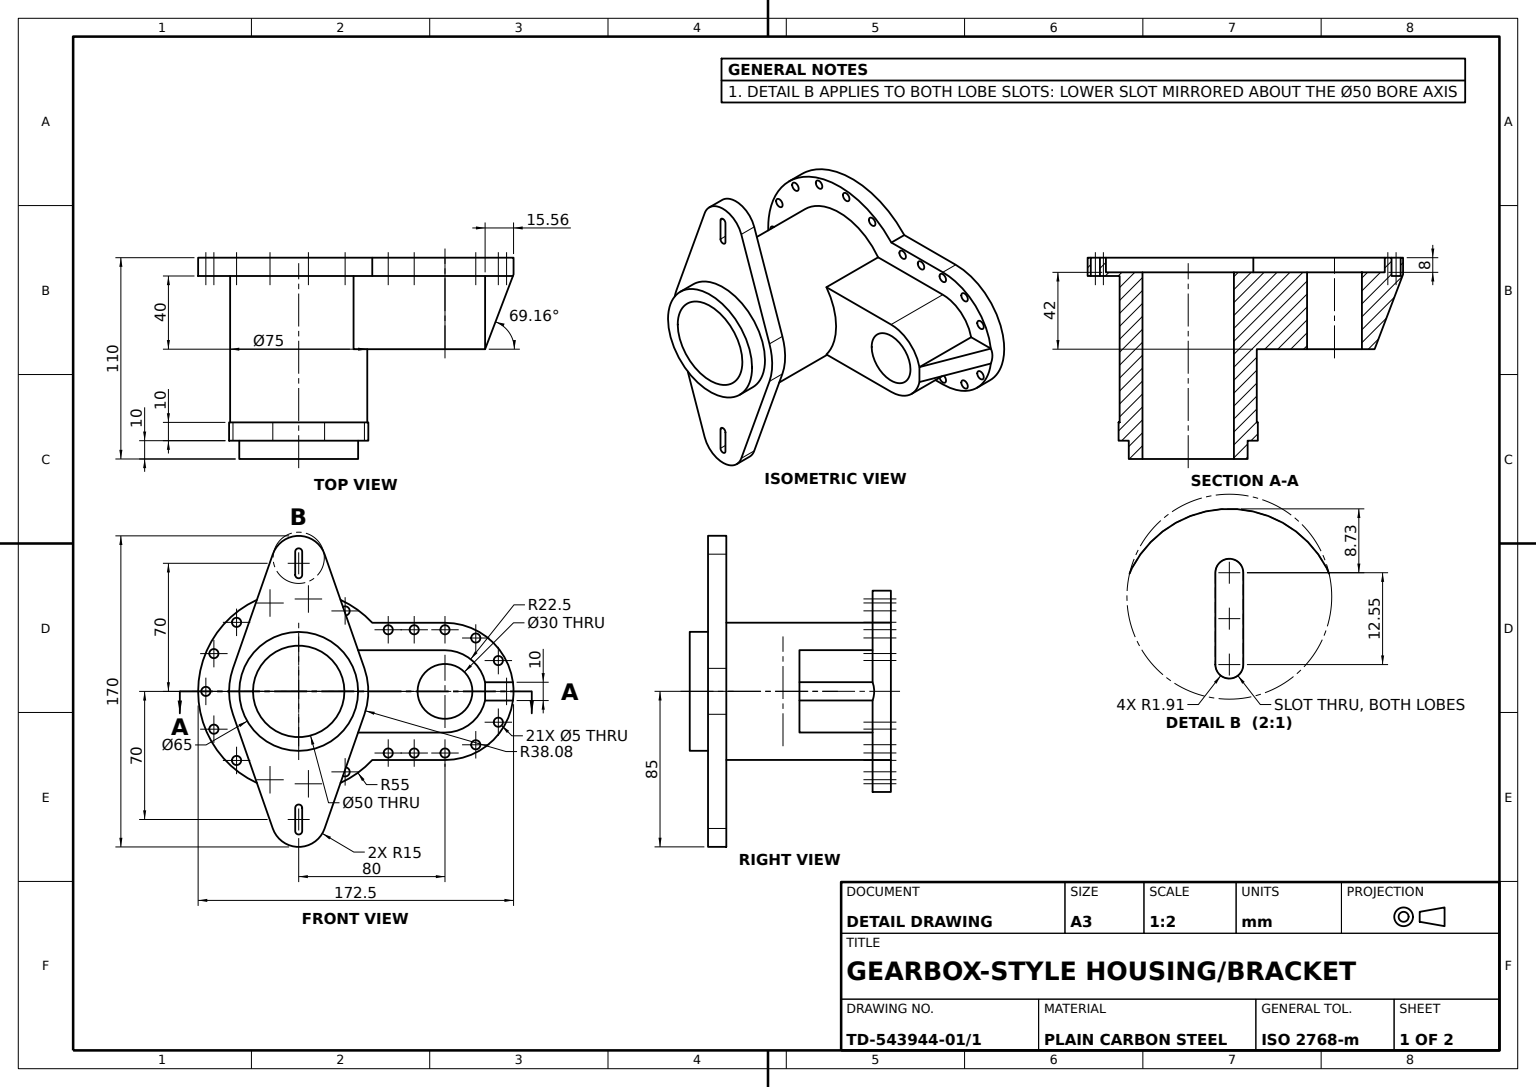
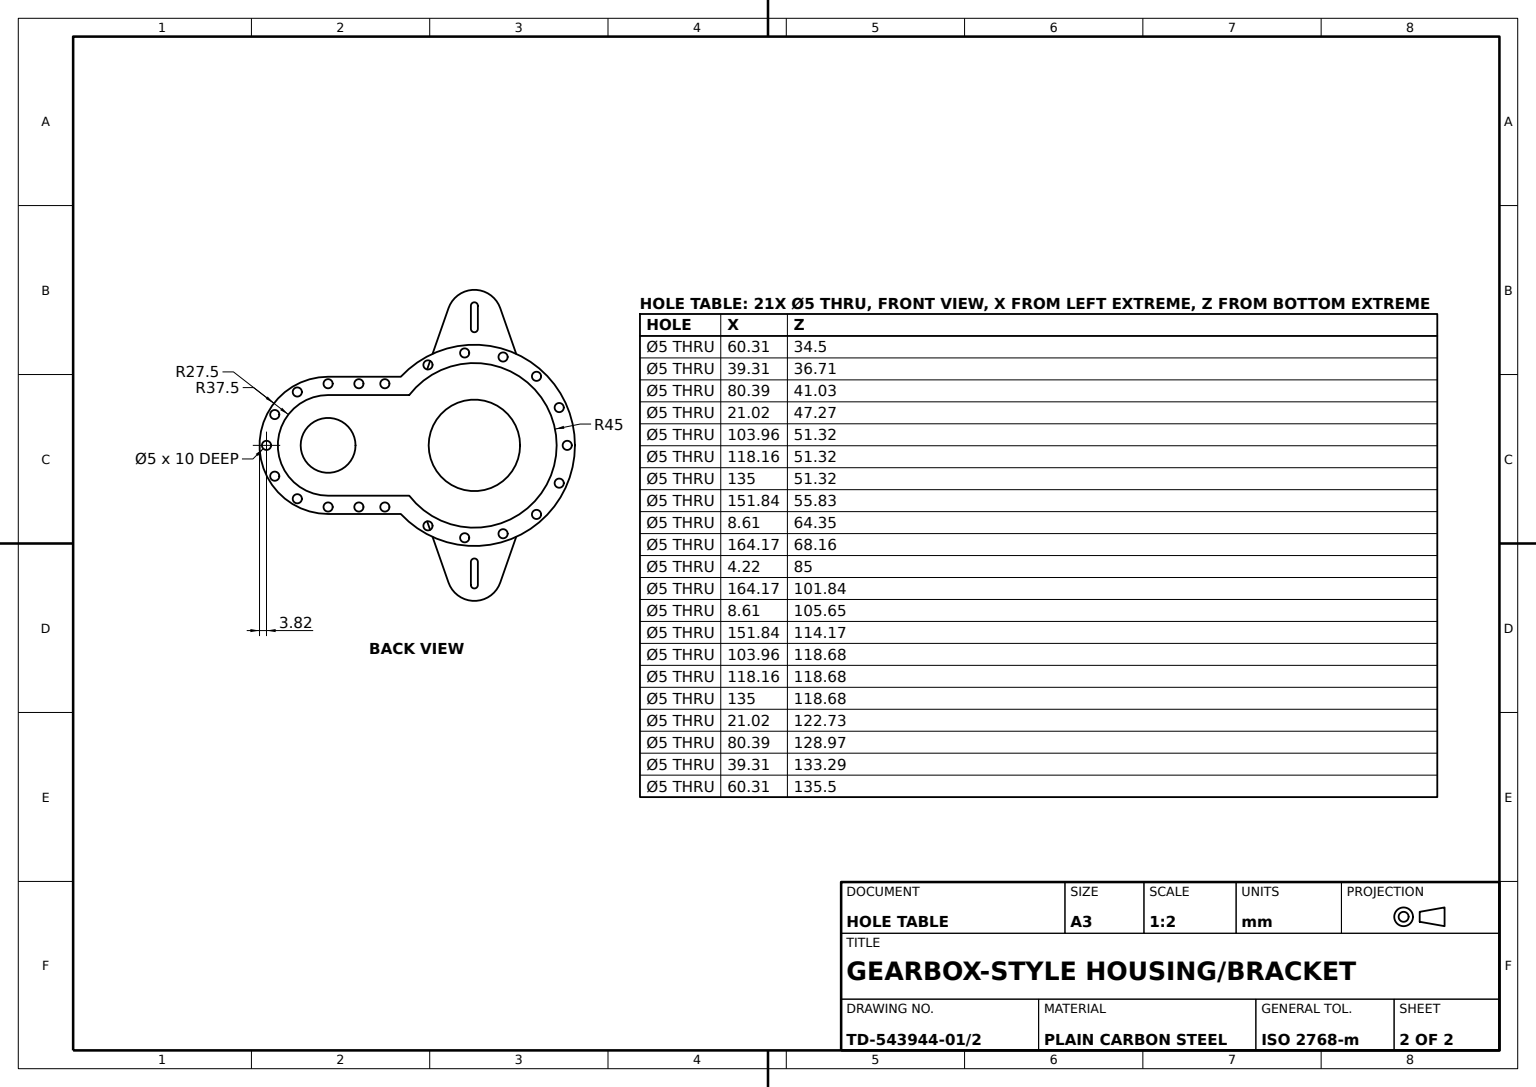
from build123d import *

# Parameters (mm, degrees)
MOUNTING_PLATE_DEPTH       = 10
BARREL_SKETCH_75_R         = 37.5
BARREL_75_DEPTH            = 80
RAISED_START               = -2
RAISED_PAD_2MM_DEPTH       = 2
END_FLANGE_DEPTH           = 10
COLLAR_AND_BORE_SKETCH_R   = 32.5
COLLAR_AND_BORE_SKETCH_R_2 = 25
BORE_COLLAR_65_DEPTH       = 10
SKETCH6_2_R                = 25
MAIN_BORE_50_DEPTH         = 177.1568903
SIDE_ARM_DEPTH             = 40
BOLT_HOLES_SKETCH_R        = 2.497943494
BOLT_HOLES_SKETCH_R_2      = 2.5
PLATE_BOLT_HOLES_DEPTH     = 40
SIDE_BORE_SKETCH_30_R      = 15
SIDE_ARM_BORE_30_DEPTH     = 70
SUPPORT_RIB_DEPTH          = 40
RIB_TRIM_CUT_DEPTH         = 185.407836059
END_FLANGE_SLOTS_DEPTH     = 177.1568903


with BuildPart() as part:
    # Mounting Plate Sketch → Mounting Plate (new body)
    with BuildSketch(Plane.XY):
        with BuildLine():
            Line((80, 37.5), (40.233692349, 37.5))
            ThreePointArc((40.233692349, 37.5), (-55, 0), (40.233692349, -37.5))
            Line((40.233692349, -37.5), (80, -37.5))
            ThreePointArc((80, -37.5), (117.5, 0), (80, 37.5))
        make_face()
        with BuildLine():
            Line((80, -27.5), (35.619517122, -27.5))
            ThreePointArc((35.619517122, -27.5), (-45, 0), (35.619517122, 27.5))
            Line((35.619517122, 27.5), (80, 27.5))
            ThreePointArc((80, 27.5), (107.5, 0), (80, -27.5))
        make_face(mode=Mode.SUBTRACT)
    extrude(amount=MOUNTING_PLATE_DEPTH)



with BuildPart() as body_2:
    # Barrel Sketch _75 → Barrel _75 (new body)
    with BuildSketch(Plane.XY.offset(10)):
        Circle(BARREL_SKETCH_75_R)
    extrude(amount=BARREL_75_DEPTH)


with BuildPart() as part_1:
    add(part.part)

    add(body_2.part)  # Raised Pad 2mm merges body 2
    # Raised Pad Sketch → Raised Pad 2mm (add)
    with BuildSketch(Plane.XY.offset(10).offset(RAISED_START)):
        with BuildLine():
            Line((35.619517122, -27.5), (80, -27.5))
            ThreePointArc((80, -27.5), (107.5, 0), (80, 27.5))
            Line((80, 27.5), (35.619517122, 27.5))
            ThreePointArc((35.619517122, 27.5), (-45, 0), (35.619517122, -27.5))
        make_face()
    extrude(amount=RAISED_PAD_2MM_DEPTH)

    # End Flange Sketch → End Flange (add)
    with BuildSketch(Plane.XY.offset(90)):
        with BuildLine():
            Line((-14.161571651, 74.944682839), (-35.946965527, 12.551314779))
            ThreePointArc((-35.946965527, 12.551314779), (-38.075186582, 0), (-35.946965527, -12.551314779))
            Line((-35.946965527, -12.551314779), (-14.161571651, -74.944682839))
            ThreePointArc((-14.161571651, -74.944682839), (0, -85), (14.161571651, -74.944682839))
            Line((14.161571651, -74.944682839), (35.946965527, -12.551314779))
            ThreePointArc((35.946965527, -12.551314779), (38.075186582, 0), (35.946965527, 12.551314779))
            Line((35.946965527, 12.551314779), (14.161571651, 74.944682839))
            ThreePointArc((14.161571651, 74.944682839), (0, 85), (-14.161571651, 74.944682839))
        make_face()
    extrude(amount=END_FLANGE_DEPTH)

    # Collar And Bore Sketch → Bore Collar _65 (add)
    with BuildSketch(Plane.XY.offset(100)):
        Circle(COLLAR_AND_BORE_SKETCH_R)
        Circle(COLLAR_AND_BORE_SKETCH_R_2, mode=Mode.SUBTRACT)
    extrude(amount=BORE_COLLAR_65_DEPTH)

    # Sketch6_2 → Main Bore _50 (cut, through all)
    with BuildSketch(Plane.XY.offset(100)):
        Circle(SKETCH6_2_R)
    extrude(amount=-MAIN_BORE_50_DEPTH, mode=Mode.SUBTRACT)

    # Side Arm Sketch → Side Arm (add)
    with BuildSketch(Plane.XY.offset(10)):
        with BuildLine():
            Line((80, 22.5), (30, 22.5))
            ThreePointArc((30, 22.5), (37.5, 0), (30, -22.5))
            Line((30, -22.5), (80, -22.5))
            ThreePointArc((80, -22.5), (102.5, 0), (80, 22.5))
        make_face()
    extrude(amount=SIDE_ARM_DEPTH)

    # Bolt Holes Sketch → Plate Bolt Holes (cut)
    with BuildSketch(Plane.XY.offset(10)):
        with Locations((63.163402703, 33.682833364)):
            Circle(BOLT_HOLES_SKETCH_R)
        with Locations((113.682833364, 0)):
            Circle(BOLT_HOLES_SKETCH_R_2)
        with Locations((109.170189364, -16.841416682)):
            Circle(BOLT_HOLES_SKETCH_R_2)
        with Locations((96.841416682, -29.170189364)):
            Circle(BOLT_HOLES_SKETCH_R_2)
        with Locations((80, -33.682833364)):
            Circle(BOLT_HOLES_SKETCH_R_2)
        with Locations((109.170189364, 16.841416682)):
            Circle(BOLT_HOLES_SKETCH_R_2)
        with Locations((80, 33.682833364)):
            Circle(BOLT_HOLES_SKETCH_R_2)
        with Locations((96.841416682, 29.170189364)):
            Circle(BOLT_HOLES_SKETCH_R_2)
        with Locations((-50.775508212, 0)):
            Circle(BOLT_HOLES_SKETCH_R_2)
        with Locations((-46.385734886, 20.652259761)):
            Circle(BOLT_HOLES_SKETCH_R_2)
        with Locations((-33.975446598, 37.733556189)):
            Circle(BOLT_HOLES_SKETCH_R_2)
        with Locations((-15.690494935, 48.290377953)):
            Circle(BOLT_HOLES_SKETCH_R_2)
        with Locations((5.307485845, 50.497354665)):
            Circle(BOLT_HOLES_SKETCH_R_2)
        with Locations((25.387754106, 43.972880001)):
            Circle(BOLT_HOLES_SKETCH_R_2)
        with Locations((25.387754106, -43.972880001)):
            Circle(BOLT_HOLES_SKETCH_R_2)
        with Locations((5.307485845, -50.497354665)):
            Circle(BOLT_HOLES_SKETCH_R_2)
        with Locations((-15.690494935, -48.290377953)):
            Circle(BOLT_HOLES_SKETCH_R_2)
        with Locations((-33.975446598, -37.733556189)):
            Circle(BOLT_HOLES_SKETCH_R_2)
        with Locations((-46.385734886, -20.652259761)):
            Circle(BOLT_HOLES_SKETCH_R_2)
        with Locations((48.957169928, 33.682833364)):
            Circle(BOLT_HOLES_SKETCH_R)
        with Locations((63.163402703, -33.682833364)):
            Circle(BOLT_HOLES_SKETCH_R)
        with Locations((48.957169928, -33.682833364)):
            Circle(BOLT_HOLES_SKETCH_R)
    extrude(amount=-PLATE_BOLT_HOLES_DEPTH, mode=Mode.SUBTRACT)

    # Side Bore Sketch _30 → Side Arm Bore _30 (cut)
    with BuildSketch(Plane.XY.offset(50)):
        with Locations((80, 0)):
            Circle(SIDE_BORE_SKETCH_30_R)
    extrude(amount=-SIDE_ARM_BORE_30_DEPTH, mode=Mode.SUBTRACT)

    # Support Rib Sketch → Support Rib (add)
    with BuildSketch(Plane.XY.offset(10)):
        with BuildLine():
            Line((101.937410968, -5), (117.165171868, -5))
            ThreePointArc((117.165171868, -5), (117.5, 0), (117.165171868, 5))
            Line((117.165171868, 5), (101.937410968, 5))
            ThreePointArc((101.937410968, 5), (102.5, 0), (101.937410968, -5))
        make_face()
    extrude(amount=SUPPORT_RIB_DEPTH)

    # Rib Trim Sketch → Rib Trim Cut (cut, through all)
    with BuildSketch(Plane.XZ.offset(5)):
        Polygon((101.937410968, 50), (130.228414001, -24.314282233), (130.228414001, 50), align=None)
    extrude(amount=-RIB_TRIM_CUT_DEPTH, mode=Mode.SUBTRACT)

    # Flange Slots Sketch → End Flange Slots (cut, through all)
    with BuildSketch(Plane.XY.offset(100)):
        with BuildLine():
            Line((1.907965824, -63.725735382), (1.907965824, -76.274264618))
            ThreePointArc((1.907965824, -76.274264618), (0, -78.182230442), (-1.907965824, -76.274264618))
            Line((-1.907965824, -76.274264618), (-1.907965824, -63.725735382))
            ThreePointArc((-1.907965824, -63.725735382), (0, -61.817769558), (1.907965824, -63.725735382))
        make_face()
        with BuildLine():
            Line((1.907965824, 63.725735382), (1.907965824, 76.274264618))
            ThreePointArc((1.907965824, 76.274264618), (0, 78.182230442), (-1.907965824, 76.274264618))
            Line((-1.907965824, 76.274264618), (-1.907965824, 63.725735382))
            ThreePointArc((-1.907965824, 63.725735382), (0, 61.817769558), (1.907965824, 63.725735382))
        make_face()
    extrude(amount=-END_FLANGE_SLOTS_DEPTH, mode=Mode.SUBTRACT)


solid = part_1.part
